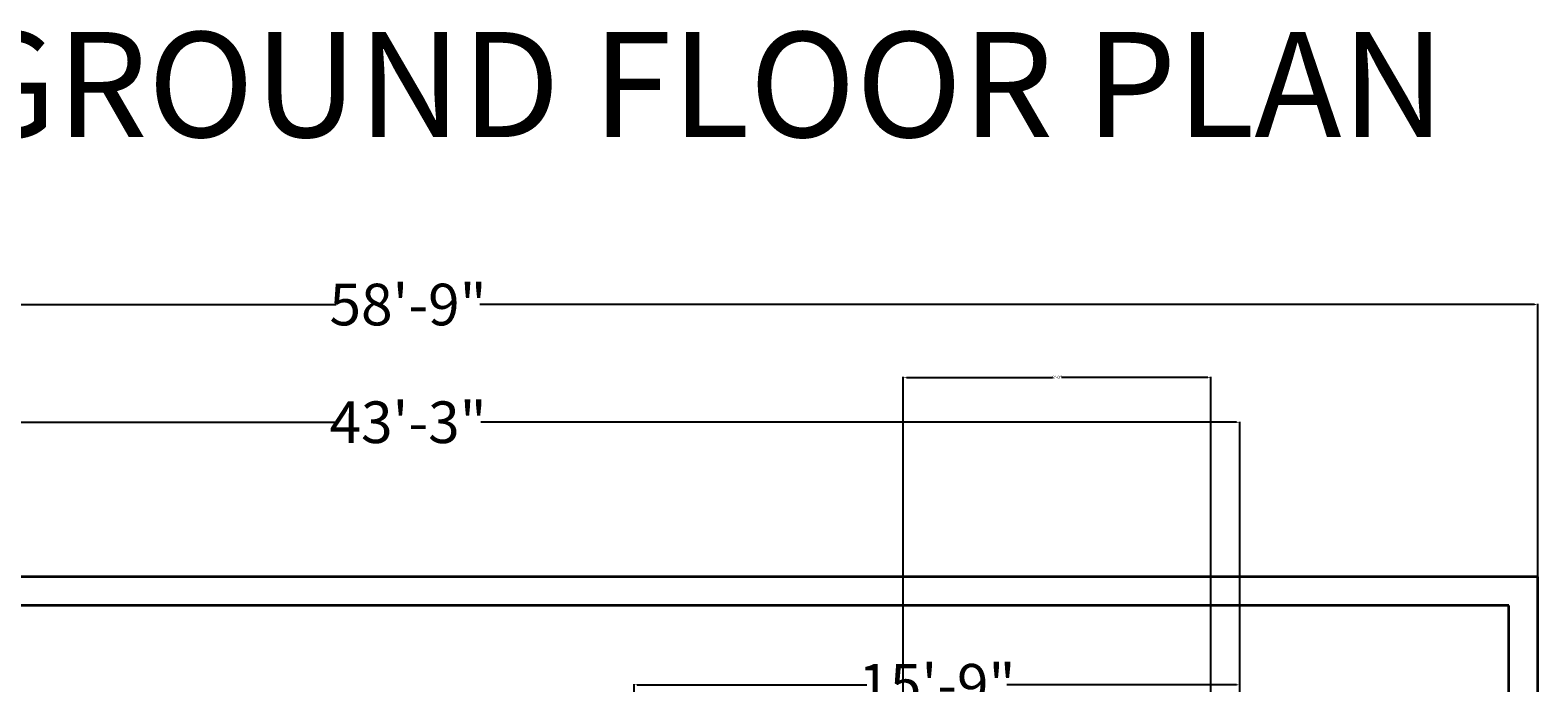
# Model space of a CAD drawing. Units: inches. Extents: x -364 to 705, y -52 to 1250.
# Tile 34 of 34: x 170 to 641, y 1046 to 1250. Entities that reach past the tile are written whole.
import ezdxf

# ---------------------------------------------------------------- set-up
doc = ezdxf.new("R2010")
doc.units = ezdxf.units.IN
doc.header["$MEASUREMENT"] = 0
for name, color, linetype, lineweight in [('A-ANNO-DIMS', 4, 'Continuous', 18), ('A-ANNO-TITL', 6, 'Continuous', 35), ('C-WALL', 41, 'Continuous', 35)]:
    doc.layers.add(name, color=color, linetype=linetype, lineweight=lineweight)
doc.styles.get("Standard").update_dxf_attribs({"font": 'arial.ttf'})
doc.dimstyles.get("Standard").update_dxf_attribs({"dimtxt": 1, "dimasz": 1, "dimexe": 0.18, "dimexo": 0.0625, "dimgap": 0.09, "dimtad": 0, "dimtih": 1, "dimtoh": 1, "dimdec": 0, "dimzin": 0, "dimdsep": 46, "dimlunit": 3, "dimtxsty": 'Standard', "dimcen": 0.09, "dimadec": 0, "dimazin": 0, "dimtfac": 1, "dimtdec": 0, "dimtofl": 0, "dimtmove": 0, "dimatfit": 3, "dimfxl": 1, "dimtolj": 1, "dimtzin": 0, "dimarcsym": 0})

# ---------------------------------------------------------------- blocks, each defined once
blk = doc.blocks.new('*D22')
at = {"layer": 'A-ANNO-DIMS', "color": 0, "lineweight": -2, "transparency": 16777216}
for p, q in [((-64.42, 1079.18), (-64.42, 1164.27)), ((-63.42, 1164.09), (265.66, 1164.09)), ((639.58, 1164.09), (310.5, 1164.09)), ((640.58, 1079.18), (640.58, 1164.27))]:
    blk.add_line(p, q, dxfattribs=at)
at = {"layer": 'A-ANNO-DIMS', "color": 0, "transparency": 16777216}
for points in [[(-63.42, 1164.26), (-63.42, 1163.93), (-64.42, 1164.09)], [(639.58, 1164.26), (639.58, 1163.93), (640.58, 1164.09)]]:
    blk.add_solid(points, dxfattribs=at)
at = {"layer": 'Defpoints', "color": 0, "transparency": 16777216}
for p in [(640.58, 1164.09), (-64.42, 1079.11), (640.58, 1079.11)]:
    blk.add_point(p, dxfattribs=at)
at = {"layer": 'A-ANNO-DIMS', "color": 0, "transparency": 16777216, "insert": (288.08, 1164.09), "char_height": 1, "attachment_point": 5}
blk.add_mtext('\\A1;{\\H13x;58\'-9"}', dxfattribs=at)
blk = doc.blocks.new('*D23')
at = {"layer": 'A-ANNO-DIMS', "color": 0, "lineweight": -2, "transparency": 16777216}
for p, q in [((28.58, 986.18), (28.58, 1127.53)), ((29.58, 1127.35), (265.4, 1127.35)), ((546.58, 1127.35), (310.76, 1127.35)), ((547.58, 986.18), (547.58, 1127.53))]:
    blk.add_line(p, q, dxfattribs=at)
at = {"layer": 'A-ANNO-DIMS', "color": 0, "transparency": 16777216}
for points in [[(29.58, 1127.52), (29.58, 1127.18), (28.58, 1127.35)], [(546.58, 1127.52), (546.58, 1127.18), (547.58, 1127.35)]]:
    blk.add_solid(points, dxfattribs=at)
at = {"layer": 'Defpoints', "color": 0, "transparency": 16777216}
for p in [(547.58, 1127.35), (28.58, 986.11), (547.58, 986.11)]:
    blk.add_point(p, dxfattribs=at)
at = {"layer": 'A-ANNO-DIMS', "color": 0, "transparency": 16777216, "insert": (288.08, 1127.35), "char_height": 1, "attachment_point": 5}
blk.add_mtext('\\A1;{\\H13x;43\'-3"}', dxfattribs=at)
blk = doc.blocks.new('*D27')
at = {"layer": 'A-ANNO-DIMS', "color": 0, "lineweight": -2, "transparency": 16777216}
for p, q in [((358.58, 986.18), (358.58, 1045.59)), ((359.58, 1045.41), (431.27, 1045.41)), ((546.58, 1045.41), (474.89, 1045.41)), ((547.58, 986.18), (547.58, 1045.59))]:
    blk.add_line(p, q, dxfattribs=at)
at = {"layer": 'A-ANNO-DIMS', "color": 0, "transparency": 16777216}
for points in [[(359.58, 1045.57), (359.58, 1045.24), (358.58, 1045.41)], [(546.58, 1045.57), (546.58, 1045.24), (547.58, 1045.41)]]:
    blk.add_solid(points, dxfattribs=at)
at = {"layer": 'Defpoints', "color": 0, "transparency": 16777216}
for p in [(547.58, 1045.41), (358.58, 986.11), (547.58, 986.11)]:
    blk.add_point(p, dxfattribs=at)
at = {"layer": 'A-ANNO-DIMS', "color": 0, "transparency": 16777216, "insert": (453.08, 1045.41), "char_height": 1, "attachment_point": 5}
blk.add_mtext('\\A1;{\\H13x;15\'-9"}', dxfattribs=at)
blk = doc.blocks.new('*D99')
at = {"layer": 'A-ANNO-DIMS', "color": 0, "lineweight": -2, "transparency": 16777216}
for p, q in [((442.58, 822.18), (442.58, 1141.54)), ((443.58, 1141.36), (489.16, 1141.36)), ((537.58, 1141.36), (492, 1141.36)), ((538.58, 822.18), (538.58, 1141.54))]:
    blk.add_line(p, q, dxfattribs=at)
at = {"layer": 'A-ANNO-DIMS', "color": 0, "transparency": 16777216}
for points in [[(443.58, 1141.53), (443.58, 1141.2), (442.58, 1141.36)], [(537.58, 1141.53), (537.58, 1141.2), (538.58, 1141.36)]]:
    blk.add_solid(points, dxfattribs=at)
at = {"layer": 'Defpoints', "color": 0, "transparency": 16777216}
for p in [(538.58, 1141.36), (442.58, 822.11), (538.58, 822.11)]:
    blk.add_point(p, dxfattribs=at)
at = {"layer": 'A-ANNO-DIMS', "color": 0, "transparency": 16777216, "insert": (490.58, 1141.36), "char_height": 1, "attachment_point": 5}
blk.add_mtext('\\A1;8\'-0"', dxfattribs=at)

msp = doc.modelspace()

# ---------------------------------------------------------------- linework, layer by layer
at = {"layer": 'C-WALL'}
for p, q in [((640.58, 1079.11), (-64.42, 1079.11)), ((640.58, 11.11), (640.58, 1079.11)), ((631.58, 1070.11), (-55.42, 1070.11)), ((631.58, 11.11), (631.58, 1070.11))]:
    msp.add_line(p, q, dxfattribs=at)

# ---------------------------------------------------------------- texts
at = {"layer": 'A-ANNO-TITL', "insert": (-74.72, 1249.15), "char_height": 32.815, "attachment_point": 1}
msp.add_mtext_dynamic_manual_height_columns('HOSPITAL GROUND FLOOR PLAN ', width=1304.1967, gutter_width=2.52, heights=[0], dxfattribs=at)

# ---------------------------------------------------------------- dimensions: what is measured, and where the dimension line sits
at = {"layer": 'A-ANNO-DIMS'}
for base, p1, p2, picture, middle in [((640.58, 1164.09), (-64.42, 1079.11), (640.58, 1079.11), '*D22', (288.08, 1164.09)), ((547.58, 1127.35), (28.58, 986.11), (547.58, 986.11), '*D23', (288.08, 1127.35)), ((547.58, 1045.41), (358.58, 986.11), (547.58, 986.11), '*D27', (453.08, 1045.41))]:
    dim = msp.add_linear_dim(base=base, p1=p1, p2=p2, text='{\\H13x;<>}', dimstyle='Standard', override={"dimclrd": 0, "dimclre": 0, "dimclrt": 0}, dxfattribs=at)
    dim.commit()
    dim.dimension.update_dxf_attribs({"geometry": picture, "text_midpoint": middle})
dim = msp.add_linear_dim(base=(538.58, 1141.36), p1=(442.58, 822.11), p2=(538.58, 822.11), dimstyle='Standard', override={"dimdec": 1, "dimlfac": 1, "dimrnd": 0, "dimzin": 1, "dimdsep": 46, "dimlunit": 4, "dimfrac": 2}, dxfattribs=at)
dim.commit()
dim.dimension.update_dxf_attribs({"geometry": '*D99', "text_midpoint": (490.58, 1141.36)})

doc.saveas('drawing.dxf')
